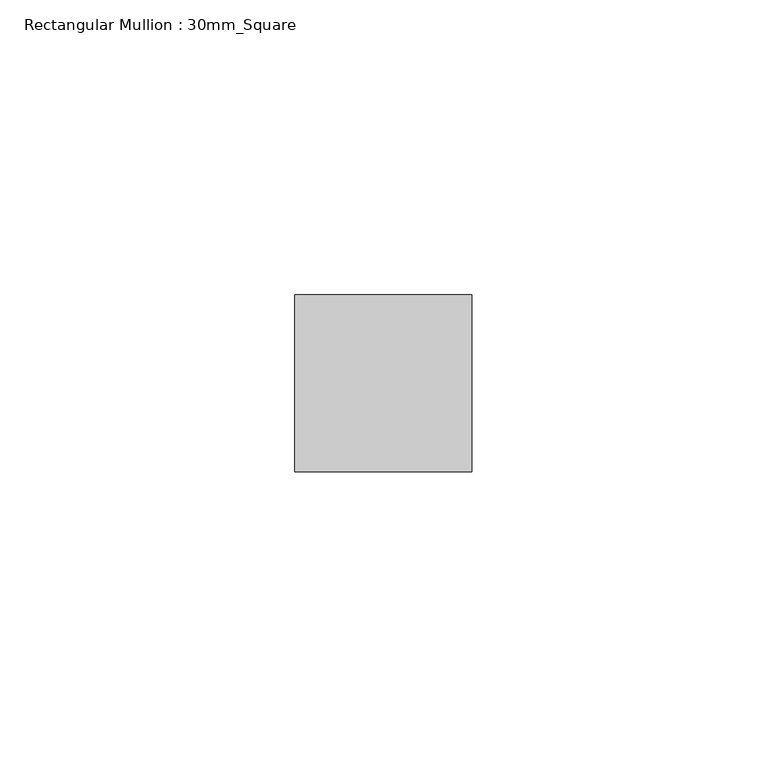
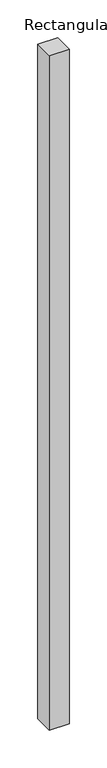
"""IFC4 building model written with IfcOpenShell, lengths in millimetres: member geometry, Rectangular Mullion : 30mm_Square."""

from ifc_helpers import new_model, si_unit, frame, origin, place, context, project, spatial, polyline, outline, extrude, source, transform, mapped, element, save


def rectangular_mullion_30mm_square_698bad25(model_context):
    return source(origin(), model_context, "Body", "SweptSolid", [
        extrude(outline(polyline([(0.0, 15.0), (0.0, -15.0), (-30.0, -15.0), (-30.0, 15.0), (0.0, 15.0)])), frame((0.0, 0.0, -1085.3), z_axis=(0.0, 0.0, 1.0), x_axis=(1.0, 0.0, 0.0)), (0.0, 0.0, 1.0), 1085.3),
    ])


if __name__ == "__main__":
    model = new_model("IFC4")
    model_context = context("Model", 3, world=origin())
    ifc_project = project(units=[si_unit("LENGTHUNIT", "METRE", prefix="MILLI")], contexts=[model_context])
    site = spatial("IfcSite", under=ifc_project)
    building = spatial("IfcBuilding", under=site)
    placement = place(None, origin())
    rectangular_mullion_30mm_square_shape = rectangular_mullion_30mm_square_698bad25(model_context)
    element("IfcMember", 1, ObjectType="Rectangular Mullion : 30mm_Square", at=placement, inside=building, context=model_context, shape_type="MappedRepresentation", body=[
        mapped(rectangular_mullion_30mm_square_shape, transform((0.0, 0.0, 0.0), x_axis=(1.0, 0.0, 0.0), y_axis=(0.0, 1.0, 0.0), z_axis=(0.0, 0.0, 1.0))),
    ])
    save(model, "model.ifc")

# Revit data of these elements
# Type "Rectangular Mullion : 30mm_Square"
#   Keynote = "H11"
#   built-in parameter 1007304 = 0.0984252 (stored number, unit not read)
#   built-in parameter 1007301 = 0.0492126 (stored number, unit not read)
#   built-in parameter 1007300 = 0.0492126 (stored number, unit not read)
# Element 1 (IfcMember, "Rectangular Mullion : 30mm_Square")
#   Materials on its faces: "Aluminium"
# Materials
#   "Aluminium": class "Metal", colour RGB 247 247 247, transparency 0, Description = "Aluminium 6061", Cost = 0
